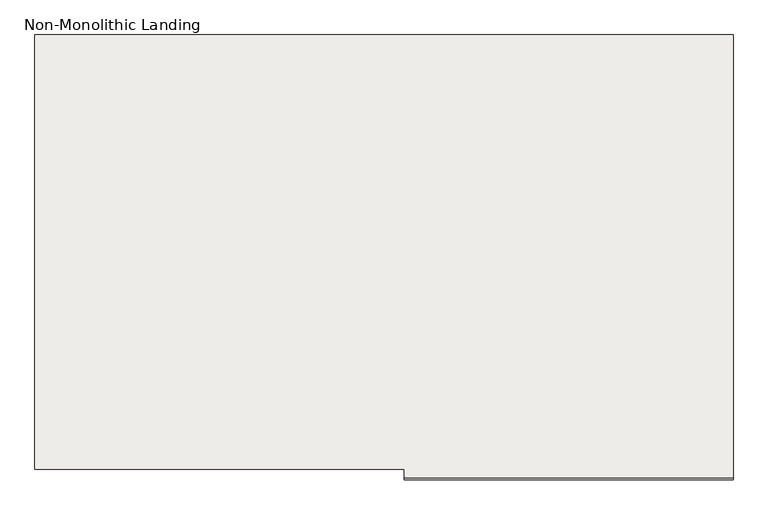
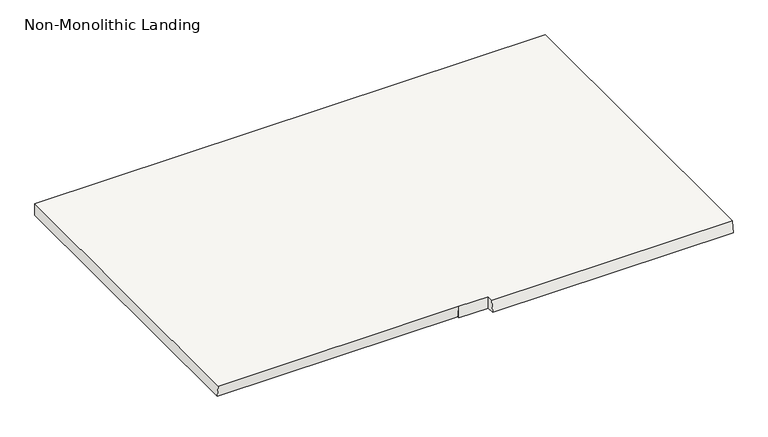
"""IFC4 building model written with IfcOpenShell, lengths in millimetres: slab geometry, Non-Monolithic Landing."""

from ifc_helpers import new_model, si_unit, origin, place, context, project, spatial, faceted_brep, source, transform, mapped, element, save


def non_monolithic_landing_64e54c11(model_context):
    return source(origin(), model_context, "Body", "Brep", [
        faceted_brep([(-3440.2939506, 10798.7482221, 1391.3043478), (-3440.2939506, 10791.5607221, 1341.3043478), (-2440.2681693, 10791.5607221, 1341.3043478), (-2440.2681693, 10798.7482221, 1391.3043478), (-3562.8939506, 10823.7482221, 1391.3043478), (-3440.2939506, 10823.7482221, 1391.3043478), (-2440.2681693, 10823.7482221, 1391.3043478), (-2440.2681693, 12144.5482221, 1391.3043478), (-4562.9197318, 12144.5482221, 1391.3043478), (-4562.9197318, 10823.7482221, 1391.3043478), (-3440.2939506, 10823.7482221, 1341.3043478), (-3562.8939506, 10823.7482221, 1341.3043478), (-3562.8939506, 10830.9357221, 1341.3043478), (-4562.9197318, 10830.9357221, 1341.3043478), (-4562.9197318, 12144.5482221, 1341.3043478), (-2440.2681693, 12144.5482221, 1341.3043478), (-2440.2681693, 10823.7482221, 1341.3043478)], [[[0, 1, 2, 3]], [[4, 5, 0, 3, 6, 7, 8, 9]], [[10, 11, 12, 13, 14, 15, 16, 2, 1]], [[5, 4, 11, 10]], [[0, 5, 10, 1]], [[6, 3, 2, 16]], [[7, 6, 16, 15]], [[8, 7, 15, 14]], [[9, 8, 14, 13]], [[4, 12, 11]], [[12, 4, 9, 13]]]),
    ])


if __name__ == "__main__":
    model = new_model("IFC4")
    model_context = context("Model", 3, world=origin())
    ifc_project = project(units=[si_unit("LENGTHUNIT", "METRE", prefix="MILLI")], contexts=[model_context])
    site = spatial("IfcSite", under=ifc_project)
    building = spatial("IfcBuilding", under=site)
    placement = place(None, origin())
    non_monolithic_landing_shape = non_monolithic_landing_64e54c11(model_context)
    element("IfcSlab", 1, ObjectType="Non-Monolithic Landing", at=placement, inside=building, context=model_context, shape_type="MappedRepresentation", body=[
        mapped(non_monolithic_landing_shape, transform((0.0, 0.0, 0.0), x_axis=(1.0, 0.0, 0.0), y_axis=(0.0, 1.0, 0.0), z_axis=(0.0, 0.0, 1.0))),
    ])
    save(model, "model.ifc")
